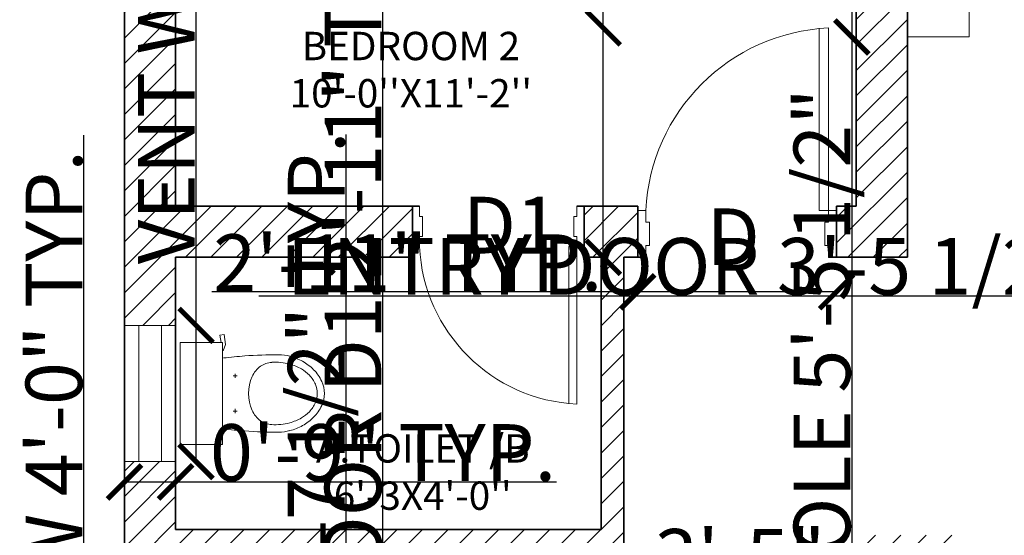
# Model space of a CAD drawing. Units: inches. Extents: x 1957 to 2456, y 1504 to 2088.
# Tile 4 of 6: x 2047 to 2220, y 1820 to 1911. Entities that reach past the tile are written whole.
import ezdxf

# ---------------------------------------------------------------- set-up
doc = ezdxf.new("R2010")
doc.units = ezdxf.units.IN
doc.header["$LTSCALE"] = 2
for name, color, linetype, lineweight in [('A-ANNO-DIMS', 2, 'Continuous', 18), ('A-ANNO-TEXT', 7, 'Continuous', 18), ('A-AREA-IDEN', 7, 'Continuous', 18), ('A-FLOR-FIXT', 8, 'Continuous', 18), ('A-FURN', 8, 'Continuous', 18), ('A-WALL-PATT', 8, 'Continuous', 13), ('Doors', 42, 'Continuous', 18), ('Walls', 7, 'Continuous', 35), ('Windows', 140, 'Continuous', 18)]:
    doc.layers.add(name, color=color, linetype=linetype, lineweight=lineweight)
doc.styles.get("Standard").update_dxf_attribs({"font": 'arial.ttf'})
doc.dimstyles.get("Standard").update_dxf_attribs({"dimtxt": 10, "dimasz": 6, "dimexe": 0.18, "dimexo": 0.0625, "dimgap": 0.09, "dimtad": 1, "dimdec": 1, "dimzin": 0, "dimdsep": 46, "dimlunit": 4, "dimtxsty": 'Standard', "dimblk": 'ARCHTICK', "dimcen": 0.09, "dimse1": 1, "dimse2": 1, "dimadec": 0, "dimazin": 0, "dimtfac": 1, "dimtdec": 1, "dimtofl": 0, "dimtmove": 0, "dimatfit": 3, "dimfxl": 1, "dimtolj": 1, "dimtzin": 0, "dimarcsym": 0})

# ---------------------------------------------------------------- blocks, each defined once
blk = doc.blocks.new('banghe81')
for p, q in [((-500, 3000), (0, 3000)), ((-500, 2312.5), (-500, 3000)), ((0, 3000), (0, 0)), ((-606.9, 1930), (-419.4, 1930)), ((-606.9, 1117.5), (-606.9, 1930)), ((-419.4, 1930), (-419.4, 1117.5)), ((-924.7, 1843.4), (-449.7, 1516.6)), ((-106.9, 1742.5), (-419.4, 1867.5)), ((-106.9, 1305), (-106.9, 1742.5)), ((-481.9, 1617.5), (-481.9, 1430)), ((-419.4, 1617.5), (-481.9, 1617.5)), ((-449.7, 1516.6), (-1057.1, 1361)), ((-481.9, 1430), (-419.4, 1430)), ((-419.4, 1180), (-106.9, 1305)), ((-419.4, 1117.5), (-606.9, 1117.5)), ((-500, 0), (-500, 687.5)), ((0, 0), (-500, 0)), ((-500, 0), (-500, 0))]:
    blk.add_line(p, q)
blk.add_arc((695.3, 1500), 1445.3, 145.79454, 214.20546)
blk = doc.blocks.new('AP0B05')
for p, q in [((35, 100), (35, 880)), ((75, 100), (75, 878.9))]:
    blk.add_line(p, q)
for points in [[(0, 100), (0, -100), (35, -100), (35, -50), (50, -50), (50, 50), (35, 50), (35, 100)], [(850, 100), (850, -100), (815, -100), (815, -50), (800, -50), (800, 50), (815, 50), (815, 100)]]:
    blk.add_lwpolyline(points, close=True)
blk.add_lwpolyline([(35, 100), (75, 100)])
blk.add_arc((-2.4, 62.6), 818.3, 2.6212, 87.3788)
blk = doc.blocks.new('_ArchTick')
at = {"color": 0, "linetype": 'ByBlock', "const_width": 0.15}
blk.add_lwpolyline([(-0.5, -0.5), (0.5, 0.5)], dxfattribs=at)
blk = doc.blocks.new('*D10')
at = {"layer": 'A-ANNO-DIMS', "color": 0, "lineweight": -2, "transparency": 16777216}
blk.add_line((2194.03, 1811.13), (2153.03, 1811.13), dxfattribs=at)
at = {"layer": 'Defpoints', "color": 0, "transparency": 16777216}
for p in [(2153.03, 1820.22), (2194.03, 1820.22), (2153.03, 1811.13)]:
    blk.add_point(p, dxfattribs=at)
at = {"layer": 'A-ANNO-DIMS', "color": 0, "lineweight": -2, "transparency": 16777216, "xscale": 6, "yscale": 6, "zscale": 6, "rotation": 180}
blk.add_blockref('_ArchTick', (2153.03, 1811.13), dxfattribs=at)
at = {"layer": 'A-ANNO-DIMS', "color": 0, "lineweight": -2, "transparency": 16777216, "xscale": 6, "yscale": 6, "zscale": 6}
blk.add_blockref('_ArchTick', (2194.03, 1811.13), dxfattribs=at)
at = {"layer": 'A-ANNO-DIMS', "color": 0, "transparency": 16777216, "insert": (2173.53, 1816.33), "char_height": 10, "attachment_point": 5}
blk.add_mtext('\\A1;3\'-5"', dxfattribs=at)
blk = doc.blocks.new('toilet-1')
at = {"color": 0, "linetype": 'ByBlock'}
for p, q in [((-0.23, -0.02), (-0.23, -0.2116)), ((0.23, -0.02), (-0.23, -0.02)), ((0.23, -0.02), (0.23, -0.2116)), ((-0.23, -0.2116), (0.23, -0.2116)), ((0.1917, -0.2144), (0.2206, -0.225)), ((0.2206, -0.225), (0.266, -0.2187)), ((0.2633, -0.1997), (0.23, -0.2044)), ((0.266, -0.2187), (0.2633, -0.1997)), ((-0.0793, -0.2587), (-0.0793, -0.2778)), ((0.0794, -0.2587), (0.0794, -0.2778)), ((-0.0889, -0.2683), (-0.0697, -0.2683)), ((0.0889, -0.2683), (0.0698, -0.2683)), ((0, -0.6382), (0, -0.6382))]:
    blk.add_line(p, q, dxfattribs=at)
for centre, radius, start, end in [((3.5272, -0.6239), 3.7093, 173.6925, 175.1593), ((-3.527, -0.624), 3.7093, 4.8413, 6.3171), ((1.7368, -0.4519), 1.9109, 175.7698, 180.3758), ((-0.0312, -0.4465), 0.1114, 113.8997, 145.1485), ((0, -0.5169), 0.1884, 66.0939, 113.9061), ((0.0312, -0.4465), 0.1114, 34.8515, 66.1003), ((-1.7366, -0.4519), 1.9109, 359.6242, 4.2302), ((-0.0408, -0.4398), 0.0996, 145.1497, 175.881), ((0.0409, -0.4398), 0.0996, 4.119, 34.8503), ((0.0981, -0.4497), 0.2389, 175.8862, 195.5931), ((-0.098, -0.4497), 0.2389, 344.4069, 4.1138), ((0.0353, -0.463), 0.2093, 180.3747, 194.3375), ((-0.0351, -0.463), 0.2093, 345.6614, 359.6243), ((0.055, -0.458), 0.2297, 194.3353, 209.622), ((0.0961, -0.4503), 0.2369, 195.5969, 209.3771), ((-0.096, -0.4503), 0.2369, 330.6229, 344.4031), ((-0.0548, -0.458), 0.2297, 330.3788, 345.6655), ((0.0647, -0.4524), 0.2409, 209.6273, 224.5489), ((0.0232, -0.4913), 0.1532, 209.3871, 226.5438), ((-0.0231, -0.4913), 0.1532, 313.4562, 330.6129), ((-0.0645, -0.4524), 0.2409, 315.4504, 330.372), ((0.0152, -0.4997), 0.1416, 226.5501, 246.5527), ((-0.0151, -0.4997), 0.1416, 293.4473, 313.4499), ((0.0178, -0.4986), 0.1751, 224.552, 245.714), ((0.0004, -0.538), 0.132, 245.5845, 269.8782), ((0, -0.5347), 0.1034, 246.5493, 270.0042), ((0, -0.5347), 0.1034, 269.9958, 293.4507), ((-0.0002, -0.538), 0.132, 270.1216, 294.4153), ((-0.0176, -0.4986), 0.1751, 294.2865, 315.4485)]:
    blk.add_arc(centre, radius, start, end, dxfattribs=at)
blk = doc.blocks.new('VENT-WIN-24IN')
for p, q in [((2.5, 0), (2.5, 24)), ((6.5, 0), (6.5, 24))]:
    blk.add_line(p, q)
blk.add_lwpolyline([(0, 0), (0, 24), (9, 24), (9, 0)], close=True)
blk = doc.blocks.new('*D17')
at = {"layer": 'A-ANNO-DIMS', "color": 0, "lineweight": -2, "transparency": 16777216}
for p, q in [((2149.43, 1909.65), (2149.43, 2059.35)), ((2149.43, 1869.22), (2149.43, 1909.65))]:
    blk.add_line(p, q, dxfattribs=at)
at = {"layer": 'Defpoints', "color": 0, "transparency": 16777216}
for p in [(2149.43, 1909.65), (2155.49, 1909.65), (2155.49, 1869.22)]:
    blk.add_point(p, dxfattribs=at)
at = {"layer": 'A-ANNO-DIMS', "color": 0, "lineweight": -2, "transparency": 16777216, "xscale": 6, "yscale": 6, "zscale": 6}
for p, rotation in [((2149.43, 1909.65), 90), ((2149.43, 1869.22), 270)]:
    blk.add_blockref('_ArchTick', p, dxfattribs=dict(at, rotation=rotation))
at = {"layer": 'A-ANNO-DIMS', "color": 0, "transparency": 16777216, "insert": (2144.16, 1987.5), "char_height": 10, "attachment_point": 5, "rotation": 90}
blk.add_mtext('\\A1;DOOR D 3\'-4 1/2" TYP.', dxfattribs=at)
blk = doc.blocks.new('*D18')
at = {"layer": 'A-ANNO-DIMS', "color": 0, "lineweight": -2, "transparency": 16777216}
for p, q in [((2155.49, 1863.15), (2080.42, 1863.15)), ((2190.56, 1863.15), (2155.49, 1863.15))]:
    blk.add_line(p, q, dxfattribs=at)
at = {"layer": 'Defpoints', "color": 0, "transparency": 16777216}
for p in [(2155.49, 1869.22), (2190.56, 1869.22), (2155.49, 1863.15)]:
    blk.add_point(p, dxfattribs=at)
at = {"layer": 'A-ANNO-DIMS', "color": 0, "lineweight": -2, "transparency": 16777216, "xscale": 6, "yscale": 6, "zscale": 6, "rotation": 180}
blk.add_blockref('_ArchTick', (2155.49, 1863.15), dxfattribs=at)
at = {"layer": 'A-ANNO-DIMS', "color": 0, "lineweight": -2, "transparency": 16777216, "xscale": 6, "yscale": 6, "zscale": 6}
blk.add_blockref('_ArchTick', (2190.56, 1863.15), dxfattribs=at)
at = {"layer": 'A-ANNO-DIMS', "color": 0, "transparency": 16777216, "insert": (2114.96, 1868.27), "char_height": 10, "attachment_point": 5}
blk.add_mtext('\\A1;2\'-11" TYP.', dxfattribs=at)
blk = doc.blocks.new('*D19')
at = {"layer": 'A-ANNO-DIMS', "color": 0, "lineweight": -2, "transparency": 16777216}
for p, q in [((2275.61, 1862.36), (2088.68, 1862.36)), ((2317.03, 1862.36), (2275.61, 1862.36))]:
    blk.add_line(p, q, dxfattribs=at)
at = {"layer": 'Defpoints', "color": 0, "transparency": 16777216}
for p in [(2275.61, 1862.36), (2275.61, 1856.15), (2317.03, 1856.15)]:
    blk.add_point(p, dxfattribs=at)
at = {"layer": 'A-ANNO-DIMS', "color": 0, "lineweight": -2, "transparency": 16777216, "xscale": 6, "yscale": 6, "zscale": 6, "rotation": 180}
blk.add_blockref('_ArchTick', (2275.61, 1862.36), dxfattribs=at)
at = {"layer": 'A-ANNO-DIMS', "color": 0, "lineweight": -2, "transparency": 16777216, "xscale": 6, "yscale": 6, "zscale": 6}
blk.add_blockref('_ArchTick', (2317.03, 1862.36), dxfattribs=at)
at = {"layer": 'A-ANNO-DIMS', "color": 0, "transparency": 16777216, "insert": (2179.14, 1867.63), "char_height": 10, "attachment_point": 5}
blk.add_mtext('\\A1;ENTRY DOOR 3\'-5 1/2" TYP.', dxfattribs=at)
blk = doc.blocks.new('*D21')
at = {"layer": 'A-ANNO-DIMS', "color": 0, "lineweight": -2, "transparency": 16777216}
for p, q in [((2110.57, 1795.08), (2110.57, 1937.02)), ((2110.57, 1760.22), (2110.57, 1795.08))]:
    blk.add_line(p, q, dxfattribs=at)
at = {"layer": 'Defpoints', "color": 0, "transparency": 16777216}
for p in [(2110.57, 1795.08), (2115.8, 1795.08), (2115.8, 1760.22)]:
    blk.add_point(p, dxfattribs=at)
at = {"layer": 'A-ANNO-DIMS', "color": 0, "lineweight": -2, "transparency": 16777216, "xscale": 6, "yscale": 6, "zscale": 6}
for p, rotation in [((2110.57, 1795.08), 90), ((2110.57, 1760.22), 270)]:
    blk.add_blockref('_ArchTick', p, dxfattribs=dict(at, rotation=rotation))
at = {"layer": 'A-ANNO-DIMS', "color": 0, "transparency": 16777216, "insert": (2105.3, 1869.05), "char_height": 10, "attachment_point": 5, "rotation": 90}
blk.add_mtext('\\A1;DOOR D1 2\'-11" TYP.', dxfattribs=at)
blk = doc.blocks.new('*D23')
at = {"layer": 'A-ANNO-DIMS', "color": 0, "lineweight": -2, "transparency": 16777216}
for p, q in [((2057.83, 1758.05), (2057.83, 1890.77)), ((2057.83, 1710.05), (2057.83, 1758.05))]:
    blk.add_line(p, q, dxfattribs=at)
at = {"layer": 'Defpoints', "color": 0, "transparency": 16777216}
for p in [(2057.83, 1758.05), (2065.03, 1758.05), (2065.03, 1710.05)]:
    blk.add_point(p, dxfattribs=at)
at = {"layer": 'A-ANNO-DIMS', "color": 0, "lineweight": -2, "transparency": 16777216, "xscale": 6, "yscale": 6, "zscale": 6}
for p, rotation in [((2057.83, 1758.05), 90), ((2057.83, 1710.05), 270)]:
    blk.add_blockref('_ArchTick', p, dxfattribs=dict(at, rotation=rotation))
at = {"layer": 'A-ANNO-DIMS', "color": 0, "transparency": 16777216, "insert": (2052.57, 1827.41), "char_height": 10, "attachment_point": 5, "rotation": 90}
blk.add_mtext('\\A1;WINDOW 4\'-0" TYP.', dxfattribs=at)
blk = doc.blocks.new('*D27')
at = {"layer": 'A-ANNO-DIMS', "color": 0, "lineweight": -2, "transparency": 16777216}
for p, q in [((2077.63, 1857.22), (2077.63, 2031.19)), ((2077.63, 1833.22), (2077.63, 1857.22))]:
    blk.add_line(p, q, dxfattribs=at)
at = {"layer": 'Defpoints', "color": 0, "transparency": 16777216}
for p in [(2074.03, 1857.22), (2077.63, 1857.22), (2074.03, 1833.22)]:
    blk.add_point(p, dxfattribs=at)
at = {"layer": 'A-ANNO-DIMS', "color": 0, "lineweight": -2, "transparency": 16777216, "xscale": 6, "yscale": 6, "zscale": 6}
for p, rotation in [((2077.63, 1857.22), 90), ((2077.63, 1833.22), 270)]:
    blk.add_blockref('_ArchTick', p, dxfattribs=dict(at, rotation=rotation))
at = {"layer": 'A-ANNO-DIMS', "color": 0, "transparency": 16777216, "insert": (2072.37, 1947.2), "char_height": 10, "attachment_point": 5, "rotation": 90}
blk.add_mtext('\\A1;VENT WINDOW 2\'-0" TYP.', dxfattribs=at)
blk = doc.blocks.new('*D28')
at = {"layer": 'A-ANNO-DIMS', "color": 0, "lineweight": -2, "transparency": 16777216}
for p, q in [((2065.03, 1829.62), (2074.03, 1829.62)), ((2074.03, 1829.62), (2141.17, 1829.62))]:
    blk.add_line(p, q, dxfattribs=at)
at = {"layer": 'Defpoints', "color": 0, "transparency": 16777216}
for p in [(2065.03, 1833.22), (2074.03, 1833.22), (2074.03, 1829.62)]:
    blk.add_point(p, dxfattribs=at)
at = {"layer": 'A-ANNO-DIMS', "color": 0, "lineweight": -2, "transparency": 16777216, "xscale": 6, "yscale": 6, "zscale": 6, "rotation": 180}
blk.add_blockref('_ArchTick', (2065.03, 1829.62), dxfattribs=at)
at = {"layer": 'A-ANNO-DIMS', "color": 0, "lineweight": -2, "transparency": 16777216, "xscale": 6, "yscale": 6, "zscale": 6}
blk.add_blockref('_ArchTick', (2074.03, 1829.62), dxfattribs=at)
at = {"layer": 'A-ANNO-DIMS', "color": 0, "transparency": 16777216, "insert": (2110.6, 1834.81), "char_height": 10, "attachment_point": 5}
blk.add_mtext('\\A1;0\'-9" TYP.', dxfattribs=at)
blk = doc.blocks.new('*D33')
at = {"layer": 'A-ANNO-DIMS', "color": 0, "lineweight": -2, "transparency": 16777216}
for p, q in [((2074.82, 1805.18), (1956.82, 1805.18)), ((2100.26, 1805.18), (2074.82, 1805.18))]:
    blk.add_line(p, q, dxfattribs=at)
at = {"layer": 'Defpoints', "color": 0, "transparency": 16777216}
for p in [(2074.82, 1805.18), (2074.82, 1801.36), (2100.26, 1801.36)]:
    blk.add_point(p, dxfattribs=at)
at = {"layer": 'A-ANNO-DIMS', "color": 0, "lineweight": -2, "transparency": 16777216, "xscale": 6, "yscale": 6, "zscale": 6, "rotation": 180}
blk.add_blockref('_ArchTick', (2074.82, 1805.18), dxfattribs=at)
at = {"layer": 'A-ANNO-DIMS', "color": 0, "lineweight": -2, "transparency": 16777216, "xscale": 6, "yscale": 6, "zscale": 6}
blk.add_blockref('_ArchTick', (2100.26, 1805.18), dxfattribs=at)
at = {"layer": 'A-ANNO-DIMS', "color": 0, "transparency": 16777216, "insert": (2012.82, 1810.44), "char_height": 10, "attachment_point": 5}
blk.add_mtext('\\A1;WC 2\'-1 1/2" TYP.', dxfattribs=at)
blk = doc.blocks.new('*D34')
at = {"layer": 'A-ANNO-DIMS', "color": 0, "lineweight": -2, "transparency": 16777216}
for p, q in [((2104.08, 1801.36), (2104.08, 1890.86)), ((2104.08, 1781.95), (2104.08, 1801.36))]:
    blk.add_line(p, q, dxfattribs=at)
at = {"layer": 'Defpoints', "color": 0, "transparency": 16777216}
for p in [(2100.26, 1801.36), (2104.08, 1801.36), (2100.26, 1781.95)]:
    blk.add_point(p, dxfattribs=at)
at = {"layer": 'A-ANNO-DIMS', "color": 0, "lineweight": -2, "transparency": 16777216, "xscale": 6, "yscale": 6, "zscale": 6}
for p, rotation in [((2104.08, 1801.36), 90), ((2104.08, 1781.95), 270)]:
    blk.add_blockref('_ArchTick', p, dxfattribs=dict(at, rotation=rotation))
at = {"layer": 'A-ANNO-DIMS', "color": 0, "transparency": 16777216, "insert": (2098.81, 1849.11), "char_height": 10, "attachment_point": 5, "rotation": 90}
blk.add_mtext('\\A1;1\'-7 1/2" TYP.', dxfattribs=at)
blk = doc.blocks.new('*D39')
at = {"layer": 'A-ANNO-DIMS', "color": 0, "lineweight": -2, "transparency": 16777216}
for p, q in [((2193.24, 1973.36), (2193.24, 1908.07)), ((2193.24, 1908.07), (2193.24, 1757.83))]:
    blk.add_line(p, q, dxfattribs=at)
at = {"layer": 'Defpoints', "color": 0, "transparency": 16777216}
for p in [(2203.03, 1973.36), (2193.24, 1908.07), (2203.03, 1908.07)]:
    blk.add_point(p, dxfattribs=at)
at = {"layer": 'A-ANNO-DIMS', "color": 0, "lineweight": -2, "transparency": 16777216, "xscale": 6, "yscale": 6, "zscale": 6}
for p, rotation in [((2193.24, 1973.36), 90), ((2193.24, 1908.07), 270)]:
    blk.add_blockref('_ArchTick', p, dxfattribs=dict(at, rotation=rotation))
at = {"layer": 'A-ANNO-DIMS', "color": 0, "transparency": 16777216, "insert": (2187.98, 1829.95), "char_height": 10, "attachment_point": 5, "rotation": 90}
blk.add_mtext('\\A1;TV CONSOLE 5\'-5 1/2"', dxfattribs=at)
blk = doc.blocks.new('*D56')
at = {"layer": 'A-ANNO-DIMS', "color": 0, "lineweight": -2, "transparency": 16777216}
blk.add_line((2040.63, 1688.22), (2040.63, 1869.22), dxfattribs=at)
at = {"layer": 'Defpoints', "color": 0, "transparency": 16777216}
for p in [(2040.63, 1869.22), (2367.03, 1869.22), (2367.03, 1688.22)]:
    blk.add_point(p, dxfattribs=at)
at = {"layer": 'A-ANNO-DIMS', "color": 0, "lineweight": -2, "transparency": 16777216, "xscale": 6, "yscale": 6, "zscale": 6}
for p, rotation in [((2040.63, 1869.22), 90), ((2040.63, 1688.22), 270)]:
    blk.add_blockref('_ArchTick', p, dxfattribs=dict(at, rotation=rotation))
at = {"layer": 'A-ANNO-DIMS', "color": 0, "transparency": 16777216, "insert": (2035.44, 1778.72), "char_height": 10, "attachment_point": 5, "rotation": 90}
blk.add_mtext('\\A1;15\'-1"', dxfattribs=at)
blk = doc.blocks.new('*D58')
at = {"layer": 'A-ANNO-DIMS', "color": 0, "lineweight": -2, "transparency": 16777216}
for p, q in [((2040.63, 1833.22), (2040.63, 1865.04)), ((2040.63, 1821.22), (2040.63, 1833.22))]:
    blk.add_line(p, q, dxfattribs=at)
at = {"layer": 'Defpoints', "color": 0, "transparency": 16777216}
for p in [(2040.63, 1833.22), (2074.03, 1833.22), (2074.03, 1821.22)]:
    blk.add_point(p, dxfattribs=at)
at = {"layer": 'A-ANNO-DIMS', "color": 0, "lineweight": -2, "transparency": 16777216, "xscale": 6, "yscale": 6, "zscale": 6}
for p, rotation in [((2040.63, 1833.22), 90), ((2040.63, 1821.22), 270)]:
    blk.add_blockref('_ArchTick', p, dxfattribs=dict(at, rotation=rotation))
at = {"layer": 'A-ANNO-DIMS', "color": 0, "transparency": 16777216, "insert": (2035.44, 1852.13), "char_height": 10, "attachment_point": 5, "rotation": 90}
blk.add_mtext('\\A1;1\'-0"', dxfattribs=at)
blk = doc.blocks.new('*D61')
at = {"layer": 'A-ANNO-DIMS', "color": 0, "lineweight": -2, "transparency": 16777216}
for p, q in [((2211.8, 2045.62), (2247.38, 2045.62)), ((2247.38, 2045.62), (2311.38, 2045.62))]:
    blk.add_line(p, q, dxfattribs=at)
at = {"layer": 'Defpoints', "color": 0, "transparency": 16777216}
for p in [(2247.38, 2045.62), (2211.8, 1820.22), (2247.38, 1820.22)]:
    blk.add_point(p, dxfattribs=at)
at = {"layer": 'A-ANNO-DIMS', "color": 0, "lineweight": -2, "transparency": 16777216, "xscale": 6, "yscale": 6, "zscale": 6, "rotation": 180}
blk.add_blockref('_ArchTick', (2211.8, 2045.62), dxfattribs=at)
at = {"layer": 'A-ANNO-DIMS', "color": 0, "lineweight": -2, "transparency": 16777216, "xscale": 6, "yscale": 6, "zscale": 6}
blk.add_blockref('_ArchTick', (2247.38, 2045.62), dxfattribs=at)
at = {"layer": 'A-ANNO-DIMS', "color": 0, "transparency": 16777216, "insert": (2282.38, 2050.88), "char_height": 10, "attachment_point": 5}
blk.add_mtext('\\A1;2\'-11 1/2"', dxfattribs=at)
blk = doc.blocks.new('*D62')
at = {"layer": 'A-ANNO-DIMS', "color": 0, "lineweight": -2, "transparency": 16777216}
for p, q in [((2074.03, 2045.62), (2108.63, 2045.62)), ((2108.63, 2045.62), (2172.63, 2045.62))]:
    blk.add_line(p, q, dxfattribs=at)
at = {"layer": 'Defpoints', "color": 0, "transparency": 16777216}
for p in [(2108.63, 2045.62), (2074.03, 1547.22), (2108.63, 1547.22)]:
    blk.add_point(p, dxfattribs=at)
at = {"layer": 'A-ANNO-DIMS', "color": 0, "lineweight": -2, "transparency": 16777216, "xscale": 6, "yscale": 6, "zscale": 6, "rotation": 180}
blk.add_blockref('_ArchTick', (2074.03, 2045.62), dxfattribs=at)
at = {"layer": 'A-ANNO-DIMS', "color": 0, "lineweight": -2, "transparency": 16777216, "xscale": 6, "yscale": 6, "zscale": 6}
blk.add_blockref('_ArchTick', (2108.63, 2045.62), dxfattribs=at)
at = {"layer": 'A-ANNO-DIMS', "color": 0, "transparency": 16777216, "insert": (2143.63, 2050.88), "char_height": 10, "attachment_point": 5}
blk.add_mtext('\\A1;2\'-10 1/2"', dxfattribs=at)
blk = doc.blocks.new('*D63')
at = {"layer": 'A-ANNO-DIMS', "color": 0, "lineweight": -2, "transparency": 16777216}
for p, q in [((2108.63, 2045.62), (2118.63, 2045.62)), ((2118.63, 2045.62), (2159.16, 2045.62))]:
    blk.add_line(p, q, dxfattribs=at)
at = {"layer": 'Defpoints', "color": 0, "transparency": 16777216}
for p in [(2118.63, 2045.62), (2108.63, 1547.22), (2118.63, 1547.22)]:
    blk.add_point(p, dxfattribs=at)
at = {"layer": 'A-ANNO-DIMS', "color": 0, "lineweight": -2, "transparency": 16777216, "xscale": 6, "yscale": 6, "zscale": 6, "rotation": 180}
blk.add_blockref('_ArchTick', (2108.63, 2045.62), dxfattribs=at)
at = {"layer": 'A-ANNO-DIMS', "color": 0, "lineweight": -2, "transparency": 16777216, "xscale": 6, "yscale": 6, "zscale": 6}
blk.add_blockref('_ArchTick', (2118.63, 2045.62), dxfattribs=at)
at = {"layer": 'A-ANNO-DIMS', "color": 0, "transparency": 16777216, "insert": (2141.89, 2050.81), "char_height": 10, "attachment_point": 5}
blk.add_mtext('\\A1;0\'-10"', dxfattribs=at)
blk = doc.blocks.new('*D68')
at = {"layer": 'A-ANNO-DIMS', "color": 0, "lineweight": -2, "transparency": 16777216}
for p, q in [((2395.43, 1821.22), (2395.43, 1853.98)), ((2395.43, 1817.22), (2395.43, 1821.22))]:
    blk.add_line(p, q, dxfattribs=at)
at = {"layer": 'Defpoints', "color": 0, "transparency": 16777216}
for p in [(2149.03, 1821.22), (2395.43, 1821.22), (2149.03, 1817.22)]:
    blk.add_point(p, dxfattribs=at)
at = {"layer": 'A-ANNO-DIMS', "color": 0, "lineweight": -2, "transparency": 16777216, "xscale": 6, "yscale": 6, "zscale": 6}
for p, rotation in [((2395.43, 1821.22), 90), ((2395.43, 1817.22), 270)]:
    blk.add_blockref('_ArchTick', p, dxfattribs=dict(at, rotation=rotation))
at = {"layer": 'A-ANNO-DIMS', "color": 0, "transparency": 16777216, "insert": (2390.24, 1840.6), "char_height": 10, "attachment_point": 5, "rotation": 90}
blk.add_mtext('\\A1;0\'-4"', dxfattribs=at)
blk = doc.blocks.new('*D69')
at = {"layer": 'A-ANNO-DIMS', "color": 0, "lineweight": -2, "transparency": 16777216}
for p, q in [((2146.03, 2045.62), (2155.49, 2045.62)), ((2155.49, 2045.62), (2211.56, 2045.62))]:
    blk.add_line(p, q, dxfattribs=at)
at = {"layer": 'Defpoints', "color": 0, "transparency": 16777216}
for p in [(2155.49, 2045.62), (2146.03, 1878.22), (2155.49, 1878.22)]:
    blk.add_point(p, dxfattribs=at)
at = {"layer": 'A-ANNO-DIMS', "color": 0, "lineweight": -2, "transparency": 16777216, "xscale": 6, "yscale": 6, "zscale": 6, "rotation": 180}
blk.add_blockref('_ArchTick', (2146.03, 2045.62), dxfattribs=at)
at = {"layer": 'A-ANNO-DIMS', "color": 0, "lineweight": -2, "transparency": 16777216, "xscale": 6, "yscale": 6, "zscale": 6}
blk.add_blockref('_ArchTick', (2155.49, 2045.62), dxfattribs=at)
at = {"layer": 'A-ANNO-DIMS', "color": 0, "transparency": 16777216, "insert": (2186.53, 2050.88), "char_height": 10, "attachment_point": 5}
blk.add_mtext('\\A1;0\'-9 1/2"', dxfattribs=at)

msp = doc.modelspace()

# ---------------------------------------------------------------- hatches: boundary and pattern name
at = {"layer": 'A-WALL-PATT', "transparency": 33554585}
h = msp.add_hatch(dxfattribs=at)
h.set_pattern_fill('ANSI31', color=256)
h.paths.add_polyline_path([(2129.18, 2021.22), (2065.03, 2021.22), (2065.03, 1857.22), (2074.03, 1857.22), (2074.03, 1869.22), (2115.8, 1869.22), (2115.8, 1878.22), (2074.03, 1878.22), (2074.03, 2012.22), (2129.18, 2012.22)])
h.paths.add_polyline_path([(2209.75, 2021.22), (2189.18, 2021.22), (2189.18, 2012.22), (2194.03, 2012.22), (2194.03, 1878.22), (2190.56, 1878.22), (2190.56, 1869.22), (2203.03, 1869.22), (2203.03, 2012.22), (2209.75, 2012.22)])
h.paths.add_polyline_path([(2273.18, 2021.22), (2245.68, 2021.22), (2245.68, 2012.22), (2273.18, 2012.22)])
h.paths.add_polyline_path([(2371.03, 2021.22), (2333.18, 2021.22), (2333.18, 2012.22), (2362.03, 2012.22), (2362.03, 1968.25), (2371.03, 1968.25)])
h.paths.add_polyline_path([(2371.03, 1869.22), (2367.03, 1869.22), (2367.03, 1546.41), (2371.03, 1546.41)])
h.paths.add_polyline_path([(2317.03, 1820.22), (2247.38, 1820.22), (2247.38, 1811.22), (2308.03, 1811.22), (2308.03, 1697.22), (2284.03, 1697.22), (2284.03, 1688.22), (2317.03, 1688.22)])
h.paths.add_polyline_path([(2236.03, 1697.22), (2203.03, 1697.22), (2203.03, 1811.22), (2211.8, 1811.22), (2211.8, 1820.22), (2194.03, 1820.22), (2194.03, 1619.22), (2074.03, 1619.22), (2074.03, 1610.22), (2203.03, 1610.22), (2203.03, 1688.22), (2236.03, 1688.22)])
h.paths.add_polyline_path([(2153.03, 1869.22), (2155.49, 1869.22), (2155.49, 1877.47), (2155.49, 1878.22), (2146.03, 1878.22), (2146.03, 1871.1), (2146.03, 1869.22), (2149.03, 1869.22), (2149.03, 1821.22), (2074.03, 1821.22), (2074.03, 1833.22), (2065.03, 1833.22), (2065.03, 1805.22), (2074.03, 1805.22), (2074.03, 1817.22), (2149.03, 1817.22), (2149.03, 1769.22), (2146.03, 1769.22), (2146.03, 1760.22), (2153.03, 1760.22), (2156.02, 1760.22), (2156.02, 1760.87), (2156.02, 1769.11), (2153.03, 1769.11)])
h.paths.add_polyline_path([(2074.03, 1781.22), (2065.03, 1781.22), (2065.03, 1758.05), (2074.03, 1758.05), (2074.03, 1760.22), (2115.8, 1760.22), (2115.8, 1767.33), (2115.8, 1769.22), (2074.03, 1769.22)])

# ---------------------------------------------------------------- linework, layer by layer
at = {"layer": 'Walls'}
for p, q in [((2065.03, 2021.22), (2065.03, 1538.22)), ((2074.03, 2012.22), (2074.03, 1878.22)), ((2194.03, 2012.22), (2194.03, 1878.22)), ((2203.03, 2012.22), (2203.03, 1869.22)), ((2117.04, 1878.22), (2074.03, 1878.22)), ((2115.8, 1878.22), (2115.8, 1869.22)), ((2155.49, 1878.22), (2144.79, 1878.22)), ((2146.03, 1869.22), (2146.03, 1878.22)), ((2155.49, 1869.22), (2155.49, 1878.22)), ((2194.03, 1878.22), (2190.56, 1878.22)), ((2190.56, 1869.22), (2190.56, 1878.22)), ((2074.03, 1869.22), (2074.03, 1821.22)), ((2115.8, 1869.22), (2074.03, 1869.22)), ((2149.03, 1869.22), (2146.03, 1869.22)), ((2149.03, 1869.22), (2149.03, 1821.22)), ((2153.03, 1869.22), (2153.03, 1769.11)), ((2156.94, 1869.22), (2153.03, 1869.22)), ((2203.03, 1869.22), (2189.12, 1869.22)), ((2149.03, 1821.22), (2074.03, 1821.22))]:
    msp.add_line(p, q, dxfattribs=at)

# ---------------------------------------------------------------- block references
at = {"layer": 'A-FLOR-FIXT', "xscale": 39.14169934857737, "yscale": 39.14169934857737, "zscale": 39.14169934857737, "rotation": 90}
msp.add_blockref('toilet-1', (2074.03, 1845.22), dxfattribs=at)
at = {"layer": 'A-FURN', "xscale": 0.0217636098217213, "yscale": 0.0217636098217213, "zscale": 0.0217636098217213, "rotation": 180}
msp.add_blockref('banghe81', (2203.03, 1973.36), dxfattribs=at)
at = {"layer": 'Doors', "xscale": -0.0412568940393612, "yscale": 0.0412568940393612, "zscale": 0.0412568940393612}
msp.add_blockref('AP0B05', (2190.56, 1873.34), dxfattribs=at)
at = {"layer": 'Doors', "xscale": 0.035574224362456, "yscale": 0.035574224362456, "zscale": 0.035574224362456, "rotation": 179.9999999999994}
msp.add_blockref('AP0B05', (2146.03, 1874.66), dxfattribs=at)
at = {"layer": 'Windows'}
msp.add_blockref('VENT-WIN-24IN', (2065.03, 1833.22), dxfattribs=at)

# ---------------------------------------------------------------- texts
at = {"layer": 'A-ANNO-TEXT'}
for s, p in [('D1', (2124.65, 1869.89)), ('D', (2167.64, 1867.84))]:
    msp.add_text(s, height=10, dxfattribs=at).set_placement(p)
at = {"layer": 'A-AREA-IDEN', "char_height": 5, "attachment_point": 1}
for s, insert in [("\\pxqc;BEDROOM 2\\P10'-0''X11'-2''", (2089.42, 1908.97)), ("\\pxqc;A.TOILET /B\\P6'-3X4'-0''", (2091.51, 1838.04))]:
    msp.add_mtext_dynamic_manual_height_columns(s, width=52.1707, gutter_width=12.5, heights=[0], dxfattribs=dict(at, insert=insert))

# ---------------------------------------------------------------- dimensions: what is measured, and where the dimension line sits
at = {"layer": 'A-ANNO-DIMS'}
for base, p1, p2, override, picture, middle in [((2108.63, 2045.62), (2074.03, 1547.22), (2108.63, 1547.22), {"dimdec": 1, "dimlfac": 1, "dimrnd": 0, "dimzin": 1, "dimdsep": 46, "dimlunit": 4, "dimfrac": 2}, '*D62', (2143.63, 2050.88)), ((2155.49, 2045.62), (2146.03, 1878.22), (2155.49, 1878.22), {"dimdec": 1, "dimlfac": 1, "dimrnd": 0, "dimzin": 1, "dimdsep": 46, "dimlunit": 4, "dimfrac": 2}, '*D69', (2186.53, 2050.88)), ((2247.38, 2045.62), (2211.8, 1820.22), (2247.38, 1820.22), {"dimdec": 1, "dimlfac": 1, "dimrnd": 0, "dimzin": 1, "dimdsep": 46, "dimlunit": 4, "dimfrac": 2}, '*D61', (2282.38, 2050.88)), ((2118.63, 2045.62), (2108.63, 1547.22), (2118.63, 1547.22), {"dimdec": 1, "dimlfac": 1, "dimrnd": 0, "dimzin": 1, "dimdsep": 46, "dimlunit": 4, "dimfrac": 2}, '*D63', (2141.89, 2050.81)), ((2153.03, 1811.13), (2194.03, 1820.22), (2153.03, 1820.22), {"dimclrd": 0, "dimclre": 0, "dimclrt": 0}, '*D10', (2173.53, 1816.33))]:
    dim = msp.add_linear_dim(base=base, p1=p1, p2=p2, dimstyle='Standard', override=override, dxfattribs=at)
    dim.commit()
    dim.dimension.update_dxf_attribs({"geometry": picture, "text_midpoint": middle})
for base, p1, p2, angle, text, picture, middle in [((2149.43, 1909.65), (2155.49, 1869.22), (2155.49, 1909.65), 90, 'DOOR D <> TYP.', '*D17', (2144.16, 1987.5)), ((2077.63, 1857.22), (2074.03, 1833.22), (2074.03, 1857.22), 90, 'VENT WINDOW <> TYP.', '*D27', (2072.37, 1947.2)), ((2193.24, 1908.07), (2203.03, 1973.36), (2203.03, 1908.07), 270, 'TV CONSOLE <>', '*D39', (2187.98, 1829.95)), ((2110.57, 1795.08), (2115.8, 1760.22), (2115.8, 1795.08), 90, 'DOOR D1 <> TYP.', '*D21', (2105.3, 1869.05)), ((2275.61, 1862.36), (2317.03, 1856.15), (2275.61, 1856.15), 180, 'ENTRY DOOR <> TYP.', '*D19', (2179.14, 1867.63)), ((2057.83, 1758.05), (2065.03, 1710.05), (2065.03, 1758.05), 90, 'WINDOW <> TYP.', '*D23', (2052.57, 1827.41)), ((2104.08, 1801.36), (2100.26, 1781.95), (2100.26, 1801.36), 90, '<> TYP.', '*D34', (2098.81, 1849.11)), ((2155.49, 1863.15), (2190.56, 1869.22), (2155.49, 1869.22), 180, '<> TYP.', '*D18', (2114.96, 1868.27)), ((2074.82, 1805.18), (2100.26, 1801.36), (2074.82, 1801.36), 180, 'WC <> TYP.', '*D33', (2012.82, 1810.44))]:
    dim = msp.add_linear_dim(base=base, p1=p1, p2=p2, angle=angle, text=text, dimstyle='Standard', override={"dimdec": 1, "dimlfac": 1, "dimrnd": 0, "dimzin": 1, "dimdsep": 46, "dimlunit": 4, "dimfrac": 2}, dxfattribs=at)
    dim.commit()
    dim.dimension.update_dxf_attribs({"geometry": picture, "text_midpoint": middle})
for base, p1, p2, picture, middle in [((2040.63, 1869.22), (2367.03, 1688.22), (2367.03, 1869.22), '*D56', (2035.44, 1778.72)), ((2040.63, 1833.22), (2074.03, 1821.22), (2074.03, 1833.22), '*D58', (2035.44, 1852.13)), ((2395.43, 1821.22), (2149.03, 1817.22), (2149.03, 1821.22), '*D68', (2390.24, 1840.6))]:
    dim = msp.add_linear_dim(base=base, p1=p1, p2=p2, angle=90, dimstyle='Standard', override={"dimdec": 1, "dimlfac": 1, "dimrnd": 0, "dimzin": 1, "dimdsep": 46, "dimlunit": 4, "dimfrac": 2}, dxfattribs=at)
    dim.commit()
    dim.dimension.update_dxf_attribs({"geometry": picture, "text_midpoint": middle})
dim = msp.add_linear_dim(base=(2074.03, 1829.62), p1=(2065.03, 1833.22), p2=(2074.03, 1833.22), text='<> TYP.', dimstyle='Standard', override={"dimdec": 1, "dimlfac": 1, "dimrnd": 0, "dimzin": 1, "dimdsep": 46, "dimlunit": 4, "dimfrac": 2}, dxfattribs=at)
dim.commit()
dim.dimension.update_dxf_attribs({"geometry": '*D28', "text_midpoint": (2110.6, 1834.81)})

doc.saveas('drawing.dxf')
